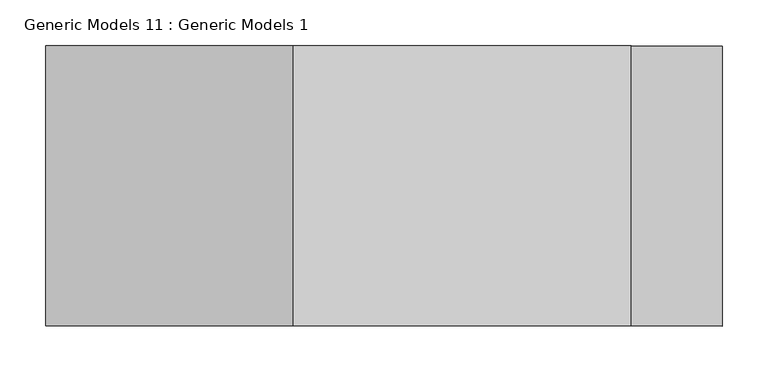
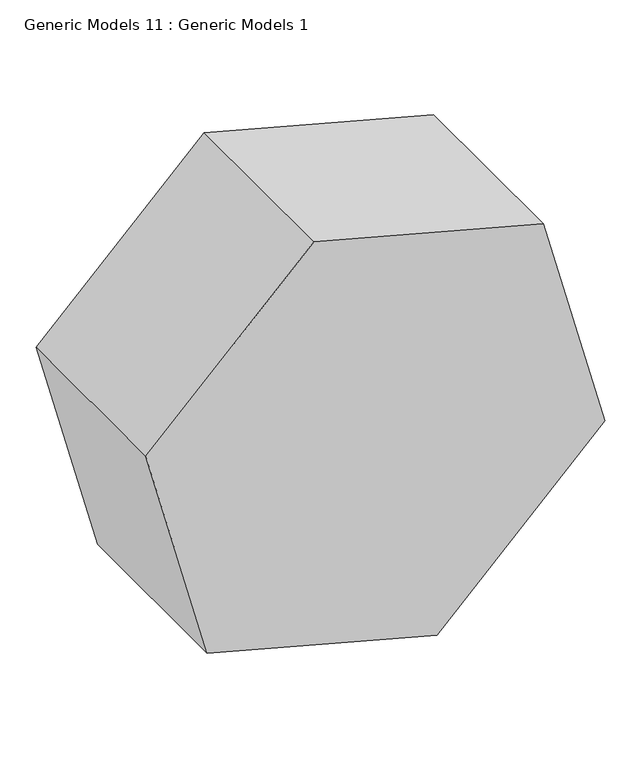
"""IFC4 building model written with IfcOpenShell, lengths in millimetres: proxy geometry, Generic Models 11 : Generic Models 1."""

from ifc_helpers import new_model, si_unit, frame, origin, place, context, project, spatial, polyline, outline, extrude, source, transform, mapped, element, save


def generic_models_11_generic_models_1_4c9ee5e0(model_context):
    return source(origin(), model_context, "Body", "SweptSolid", [
        extrude(outline(polyline([(904.7566299, 2421.0198357), (1003.366686, 2053.0020959), (733.9590024, 1783.5944123), (365.9412626, 1882.2044685), (267.3312064, 2250.2222083), (536.73889, 2519.6298919), (904.7566299, 2421.0198357)])), frame((0.0, -9086.6225464, 0.0), z_axis=(0.0, 1.0, 0.0), x_axis=(0.0, 0.0, 1.0)), (0.0, 0.0, 1.0), 304.8),
    ])


if __name__ == "__main__":
    model = new_model("IFC4")
    model_context = context("Model", 3, world=origin())
    ifc_project = project(units=[si_unit("LENGTHUNIT", "METRE", prefix="MILLI")], contexts=[model_context])
    site = spatial("IfcSite", under=ifc_project)
    building = spatial("IfcBuilding", under=site)
    placement = place(None, origin())
    generic_models_11_generic_models_1_shape = generic_models_11_generic_models_1_4c9ee5e0(model_context)
    element("IfcBuildingElementProxy", 1, Name="Generic Models 11 : Generic Models 1", ObjectType="Generic Models 11 : Generic Models 1", at=placement, inside=building, context=model_context, shape_type="MappedRepresentation", body=[
        mapped(generic_models_11_generic_models_1_shape, transform((0.0, 0.0, 0.0), x_axis=(1.0, 0.0, 0.0), y_axis=(0.0, 1.0, 0.0), z_axis=(0.0, 0.0, 1.0))),
    ])
    save(model, "model.ifc")

# Revit data of these elements
# Element 1 (IfcBuildingElementProxy, "Generic Models 11 : Generic Models 1")
#   Materials on its faces: "Carpet (1)"
# Materials
#   "Carpet (1)": class "Carpet", colour RGB 124 80 67, transparency 0, Description = "Interior finish", Cost = 0
